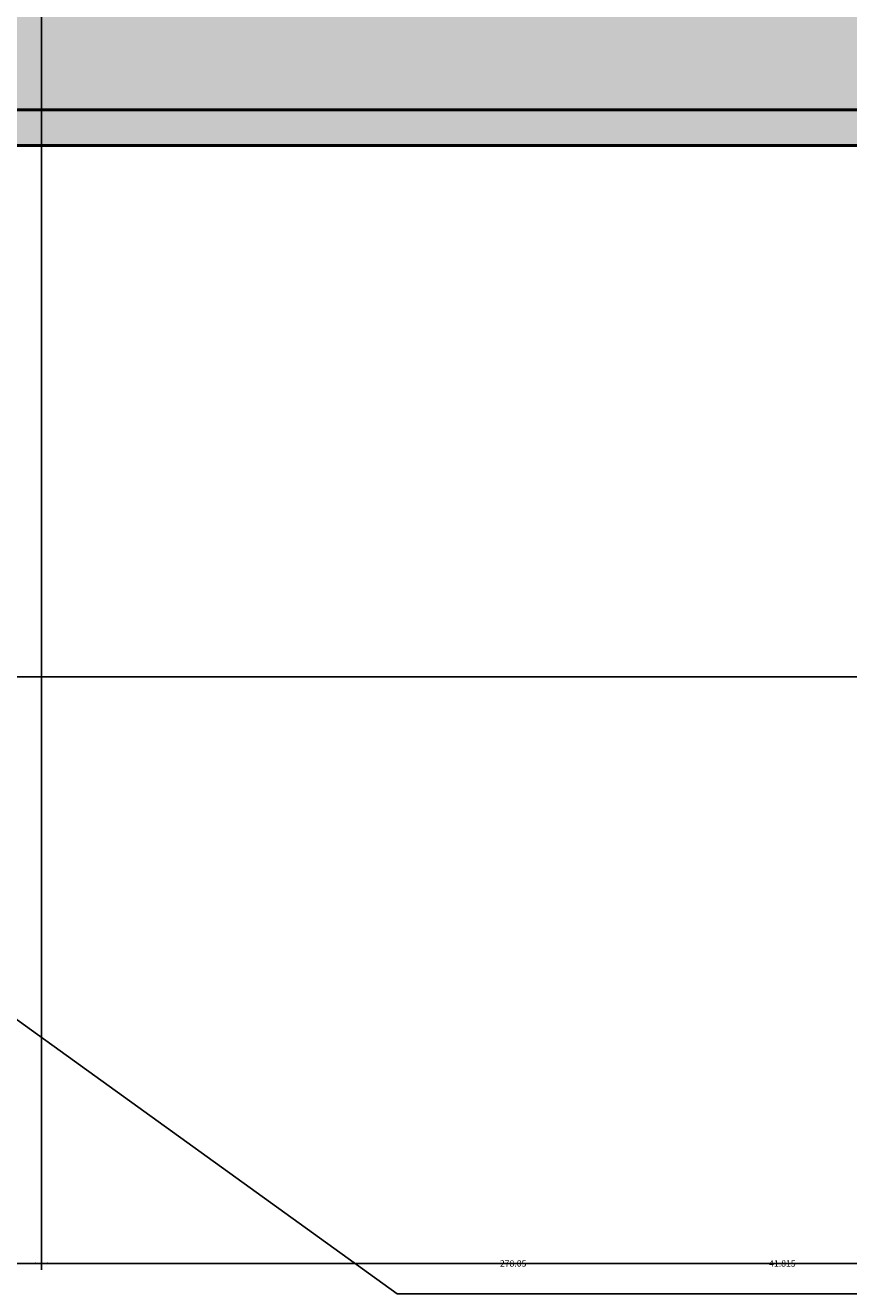
# Model space of a CAD drawing. Units: inches. Extents: x -12 to 334, y -10 to 186.
# Tile 31 of 77: x 129 to 152, y 14 to 49. Entities that reach past the tile are written whole.
import ezdxf
from ezdxf import colors
from ezdxf.entities.mleader import LeaderData, LeaderLine
from ezdxf.math import Vec2, Vec3

# ---------------------------------------------------------------- set-up
doc = ezdxf.new("R2010")
doc.units = ezdxf.units.IN
doc.header["$MEASUREMENT"] = 0
for name, color, linetype, lineweight in [('M-ANNO-TEXT', 3, 'Continuous', 25), ('M-DIMS', 2, 'Continuous', 18), ('M-EQPM', 7, 'Continuous', 50), ('M-EQPM-PATT', 8, 'Continuous', 18)]:
    doc.layers.add(name, color=color, linetype=linetype, lineweight=lineweight)
doc.styles.get("Standard").update_dxf_attribs({"font": 'arial.ttf'})
doc.dimstyles.get("Standard").update_dxf_attribs({"dimtxt": 0.18, "dimasz": 0.18, "dimexe": 0.18, "dimexo": 0.0625, "dimgap": 0.09, "dimtad": 0, "dimtih": 1, "dimtoh": 1, "dimdec": 4, "dimzin": 0, "dimdsep": 46, "dimtxsty": 'Standard', "dimcen": 0.09, "dimadec": 0, "dimazin": 0, "dimtfac": 1, "dimtdec": 4, "dimtofl": 0, "dimtmove": 0, "dimatfit": 3, "dimfxl": 1, "dimtolj": 1, "dimtzin": 0, "dimarcsym": 0})

# ---------------------------------------------------------------- blocks, each defined once
blk = doc.blocks.new('*D1')
at = {"layer": 'Defpoints', "color": 0, "transparency": 16777216}
for p in [(281.426, 91.899), (3.376, 80.692), (281.426, 14.304)]:
    blk.add_point(p, dxfattribs=at)
at = {"layer": 'M-DIMS', "color": 0, "lineweight": -2, "transparency": 16777216}
for p, q in [((281.426, 91.836), (281.426, 14.124)), ((3.376, 80.629), (3.376, 14.124)), ((3.556, 14.304), (141.935, 14.304)), ((281.246, 14.304), (142.867, 14.304))]:
    blk.add_line(p, q, dxfattribs=at)
at = {"layer": 'M-DIMS', "color": 0, "transparency": 16777216}
for points in [[(3.556, 14.334), (3.556, 14.274), (3.376, 14.304)], [(281.246, 14.334), (281.246, 14.274), (281.426, 14.304)]]:
    blk.add_solid(points, dxfattribs=at)
at = {"layer": 'M-DIMS', "color": 0, "transparency": 16777216, "insert": (142.401, 14.304), "char_height": 0.18, "attachment_point": 5}
blk.add_mtext('\\A1;278.05', dxfattribs=at)
blk = doc.blocks.new('*D29')
at = {"layer": 'Defpoints', "color": 0, "transparency": 16777216}
for p in [(-11.174, 45.854), (221.576, 45.854), (216.576, 30.854)]:
    blk.add_point(p, dxfattribs=at)
at = {"layer": 'M-DIMS', "color": 0, "lineweight": -2, "transparency": 16777216}
for p, q in [((221.514, 45.854), (-11.354, 45.854)), ((-11.174, 45.674), (-11.174, 38.536)), ((-11.174, 31.034), (-11.174, 38.172)), ((216.514, 30.854), (-11.354, 30.854))]:
    blk.add_line(p, q, dxfattribs=at)
at = {"layer": 'M-DIMS', "color": 0, "transparency": 16777216}
for points in [[(-11.204, 45.674), (-11.144, 45.674), (-11.174, 45.854)], [(-11.204, 31.034), (-11.144, 31.034), (-11.174, 30.854)]]:
    blk.add_solid(points, dxfattribs=at)
at = {"layer": 'M-DIMS', "color": 0, "transparency": 16777216, "insert": (-11.174, 38.354), "char_height": 0.18, "attachment_point": 5}
blk.add_mtext('\\A1;15', dxfattribs=at)
blk = doc.blocks.new('*D30')
at = {"layer": 'Defpoints', "color": 0, "transparency": 16777216}
for p in [(75.924, 63.612), (129.093, 61.105), (129.093, 14.304)]:
    blk.add_point(p, dxfattribs=at)
at = {"layer": 'M-DIMS', "color": 0, "lineweight": -2, "transparency": 16777216}
for p, q in [((75.924, 63.549), (75.924, 14.124)), ((129.093, 61.042), (129.093, 14.124)), ((76.104, 14.304), (102.115, 14.304)), ((128.913, 14.304), (102.902, 14.304))]:
    blk.add_line(p, q, dxfattribs=at)
at = {"layer": 'M-DIMS', "color": 0, "transparency": 16777216}
for points in [[(76.104, 14.334), (76.104, 14.274), (75.924, 14.304)], [(128.913, 14.334), (128.913, 14.274), (129.093, 14.304)]]:
    blk.add_solid(points, dxfattribs=at)
at = {"layer": 'M-DIMS', "color": 0, "transparency": 16777216, "insert": (102.509, 14.304), "char_height": 0.18, "attachment_point": 5}
blk.add_mtext('\\A1;53.17', dxfattribs=at)
blk = doc.blocks.new('*D31')
at = {"layer": 'Defpoints', "color": 0, "transparency": 16777216}
for p in [(129.093, 61.105), (170.908, 61.105), (170.908, 14.304)]:
    blk.add_point(p, dxfattribs=at)
at = {"layer": 'M-DIMS', "color": 0, "lineweight": -2, "transparency": 16777216}
for p, q in [((129.093, 61.042), (129.093, 14.124)), ((170.908, 61.042), (170.908, 14.124)), ((129.273, 14.304), (149.532, 14.304)), ((170.728, 14.304), (150.468, 14.304))]:
    blk.add_line(p, q, dxfattribs=at)
at = {"layer": 'M-DIMS', "color": 0, "transparency": 16777216}
for points in [[(129.273, 14.334), (129.273, 14.274), (129.093, 14.304)], [(170.728, 14.334), (170.728, 14.274), (170.908, 14.304)]]:
    blk.add_solid(points, dxfattribs=at)
at = {"layer": 'M-DIMS', "color": 0, "transparency": 16777216, "insert": (150, 14.304), "char_height": 0.18, "attachment_point": 5}
blk.add_mtext('\\A1;41.815', dxfattribs=at)
blk = doc.blocks.new('*D39')
at = {"layer": 'Defpoints', "color": 0, "transparency": 16777216}
for p in [(279.726, 80.692), (-11.174, 45.854), (269.381, 45.854)]:
    blk.add_point(p, dxfattribs=at)
at = {"layer": 'M-DIMS', "color": 0, "lineweight": -2, "transparency": 16777216}
for p, q in [((279.664, 80.692), (-11.354, 80.692)), ((-11.174, 80.512), (-11.174, 63.455)), ((-11.174, 46.034), (-11.174, 63.091)), ((269.318, 45.854), (-11.354, 45.854))]:
    blk.add_line(p, q, dxfattribs=at)
at = {"layer": 'M-DIMS', "color": 0, "transparency": 16777216}
for points in [[(-11.204, 80.512), (-11.144, 80.512), (-11.174, 80.692)], [(-11.204, 46.034), (-11.144, 46.034), (-11.174, 45.854)]]:
    blk.add_solid(points, dxfattribs=at)
at = {"layer": 'M-DIMS', "color": 0, "transparency": 16777216, "insert": (-11.174, 63.273), "char_height": 0.18, "attachment_point": 5}
blk.add_mtext('\\A1;34.84', dxfattribs=at)

msp = doc.modelspace()

# ---------------------------------------------------------------- hatches: boundary and pattern name
at = {"layer": 'M-EQPM-PATT'}
h = msp.add_hatch(color=256, dxfattribs=at)
h.set_gradient(color1=(99, 100, 102), color2=(99, 100, 102), tint=1)
h.paths.add_polyline_path([(4.3766, 80.754, -0.4132606), (23.5807, 99.8958), (37.1002, 99.8958), (37.1002, 127.7078), (32.1002, 127.7078), (32.1002, 125.2078), (36.1002, 125.2078), (36.1002, 100.8958), (23.5807, 100.8958, 1), (23.5807, 60.4872), (36.1002, 60.4872), (36.1002, 36.1752), (32.1002, 36.1752), (32.1002, 33.6752), (37.1002, 33.6752), (37.1002, 61.4872), (23.5807, 61.4872, -0.384914), (4.4744, 78.754), (72.9244, 78.754), (72.9244, 69.6117), (75.9244, 69.6117), (75.9244, 89.8963), (72.9244, 89.8963), (72.9244, 80.754)])
h.paths.add_polyline_path([(54.1002, 125.2078), (58.1002, 125.2078), (58.1002, 127.7078), (53.1002, 127.7078), (53.1002, 99.8958), (64.5, 99.8958), (64.5, 109.0583), (63.5, 109.0583), (63.5, 100.8958), (54.1002, 100.8958)], flags=17)
h.paths.add_polyline_path([(53.1002, 33.6752), (58.1002, 33.6752), (58.1002, 36.1752), (54.1002, 36.1752), (54.1002, 60.4872), (64.2068, 60.4872), (64.2068, 49.4497), (87.8879, 49.4497), (87.8879, 55.3205), (104.8919, 55.3205), (104.8919, 30.8541), (99.8919, 30.8541), (99.8919, 28.8541), (105.8919, 28.8541), (105.8919, 56.3205), (87.8879, 56.3205), (87.8879, 63.6117), (86.8879, 63.6117), (86.8879, 50.4497), (65.0061, 50.4497), (65.0061, 63.6117), (64.5, 63.6117), (64.5, 61.4872), (53.1002, 61.4872)])
h.paths.add_polyline_path([(121.8919, 28.8541), (121.8919, 30.8541), (116.8919, 30.8541), (116.8919, 45.8541), (209.6965, 45.8541), (209.9204, 46.8541), (115.8919, 46.8541), (115.8919, 28.8541)])
h.paths.add_polyline_path([(221.5761, 32.8541), (216.5761, 32.8541), (216.5761, 30.8541), (222.5761, 30.8541), (222.5761, 46.8541), (209.9204, 46.8541), (209.6965, 45.8541), (221.5761, 45.8541)])
h.paths.add_polyline_path([(233.5761, 45.8541), (249.8485, 45.8541), (249.3759, 46.8541), (232.5761, 46.8541), (232.5761, 30.8541), (238.5761, 30.8541), (238.5761, 32.8541), (233.5761, 32.8541)])
h = msp.add_hatch(color=256, dxfattribs=at)
h.set_gradient(color1=(94, 103, 175), color2=(94, 103, 175), tint=1)
h.paths.add_polyline_path([(129.093, 89.8963), (86.8879, 89.8963), (86.8879, 69.6117), (129.093, 69.6117)], flags=17)
h.paths.add_polyline_path([(170.9079, 89.8963), (130.8573, 89.8963), (130.8573, 69.6117), (170.9079, 69.6117)], flags=17)
h.paths.add_polyline_path([(216.4278, 89.8963), (172.6722, 89.8963), (172.6722, 69.6117), (216.4278, 69.6117)], flags=17)
h.paths.add_polyline_path([(245.9354, 82.6969), (247.9354, 82.6969), (247.9354, 46.8541), (268.3808, 46.8541, 0.0998398), (279.7263, 80.6915), (251.9801, 80.6915, 0.4142136), (231.7758, 100.8958), (84.7229, 100.8958), (84.7229, 109.0583), (83.7229, 109.0583), (83.7229, 95.8963), (129.093, 95.8963), (129.093, 98.1081), (130.8573, 98.1081), (130.8573, 95.8963), (170.9079, 95.8963), (170.9079, 98.1081), (172.6722, 98.1081), (172.6722, 95.8963), (216.4278, 95.8963), (216.4278, 98.1081), (218.1922, 98.1081), (218.1922, 95.8963), (226.6083, 95.8963, -1), (226.6083, 63.6117), (218.1922, 63.6117), (218.1922, 61.1045), (216.4278, 61.1045), (216.4278, 63.6117), (172.6722, 63.6117), (172.6722, 61.1045), (170.9079, 61.1045), (170.9079, 63.6117), (130.8573, 63.6117), (130.8573, 61.1045), (129.093, 61.1045), (129.093, 63.6117), (87.8879, 63.6117), (87.8879, 56.3205), (105.8919, 56.3205), (105.8919, 28.8541), (115.8919, 28.8541), (115.8919, 46.8541), (222.5761, 46.8541), (222.5761, 30.8541), (232.5761, 30.8541), (232.5761, 46.8541), (245.9354, 46.8541)])
h.paths.add_polyline_path([(86.8879, 89.8963), (75.9244, 89.8963), (75.9244, 69.6117), (86.8879, 69.6117)])
h.paths.add_polyline_path([(83.7229, 109.0583), (75.9244, 109.0583), (75.9244, 95.8963), (83.7229, 95.8963)])
h.paths.add_polyline_path([(226.6083, 89.8963), (218.1922, 89.8963), (218.1922, 69.6117), (226.6083, 69.6117, 1)], flags=17)
h = msp.add_hatch(color=256, dxfattribs=at)
h.set_gradient(color1=(0, 0, 255), color2=(0, 0, 255), tint=1)
h.paths.add_polyline_path([(84.7229, 100.8958), (84.7229, 109.0583), (83.7229, 109.0583), (83.7229, 95.8963), (129.093, 95.8963), (129.093, 98.1081), (130.8573, 98.1081), (130.8573, 95.8963), (170.9079, 95.8963), (170.9079, 98.1081), (172.6722, 98.1081), (172.6722, 95.8963), (216.4278, 95.8963), (216.4278, 98.1081), (218.1922, 98.1081), (218.1922, 95.8963), (226.6083, 95.8963, -1), (226.6083, 63.6117), (218.1922, 63.6117), (218.1922, 61.1045), (216.4278, 61.1045), (216.4278, 63.6117), (172.6722, 63.6117), (172.6722, 61.1045), (170.9079, 61.1045), (170.9079, 63.6117), (130.8573, 63.6117), (130.8573, 61.1045), (129.093, 61.1045), (129.093, 63.6117), (87.8879, 63.6117), (87.8879, 56.3205), (105.8919, 56.3205), (105.8919, 28.8541), (115.8919, 28.8541), (115.8919, 46.8541), (222.5761, 46.8541), (222.5761, 30.8541), (232.5761, 30.8541), (232.5761, 46.8541), (245.9354, 46.8541), (245.9354, 82.6969), (247.9354, 82.6969), (247.9354, 46.8541), (268.3808, 46.8541, 0.0998398), (279.7263, 80.6915), (251.9801, 80.6915, 0.4142136), (231.7758, 100.8958)])

# ---------------------------------------------------------------- linework, layer by layer
at = {"layer": 'M-EQPM'}
for p, q in [((222.5761, 46.8541), (115.8919, 46.8541)), ((221.5761, 45.8541), (116.8919, 45.8541))]:
    msp.add_line(p, q, dxfattribs=at)

# ---------------------------------------------------------------- dimensions: what is measured, and where the dimension line sits
at = {"layer": 'M-DIMS'}
for base, p1, p2, override, picture, middle in [((281.4256, 14.3041), (3.3765, 80.6915), (281.4256, 91.8988), {"dimdec": 2, "dimlfac": 1, "dimrnd": 0, "dimzin": 0, "dimdsep": 46, "dimlunit": 2}, '*D1', (142.401, 14.3041)), ((129.093, 14.3041), (75.9244, 63.6117), (129.093, 61.1045), {"dimdec": 2, "dimlfac": 1, "dimrnd": 0, "dimzin": 0, "dimdsep": 46, "dimlunit": 2}, '*D30', (102.5087, 14.3041)), ((170.9079, 14.3041), (129.093, 61.1045), (170.9079, 61.1045), {"dimdec": 3, "dimlfac": 1, "dimrnd": 0, "dimzin": 0, "dimdsep": 46, "dimlunit": 2}, '*D31', (150.0004, 14.3041))]:
    dim = msp.add_linear_dim(base=base, p1=p1, p2=p2, dimstyle='Standard', override=override, dxfattribs=at)
    dim.commit()
    dim.dimension.update_dxf_attribs({"geometry": picture, "text_midpoint": middle})
for p1, p2, override, picture, middle in [((279.7263, 80.6915), (269.3808, 45.8541), {"dimdec": 2, "dimlfac": 1, "dimrnd": 0, "dimzin": 0, "dimdsep": 46, "dimlunit": 2}, '*D39', (-11.1735, 63.2728)), ((216.5761, 30.8541), (221.5761, 45.8541), {"dimdec": 0, "dimlfac": 1, "dimrnd": 0, "dimzin": 0, "dimdsep": 46, "dimlunit": 2}, '*D29', (-11.1735, 38.3541))]:
    dim = msp.add_linear_dim(base=(-11.1736, 45.8541), p1=p1, p2=p2, angle=90, dimstyle='Standard', override=override, dxfattribs=at)
    dim.commit()
    dim.dimension.update_dxf_attribs({"geometry": picture, "text_midpoint": middle})

# ---------------------------------------------------------------- leaders
at = {"layer": 'M-ANNO-TEXT'}
ml = msp.add_multileader_mtext('Standard', dxfattribs=at)
ml.set_content('^ICondensate outlet', color=256)
ml.set_leader_properties()
ml.build(insert=Vec2(0, 0))
ml.multileader.update_dxf_attribs({"dogleg_length": 0.36, "arrow_head_size": 0.7})
ctx = ml.context
ctx.base_point, ctx.arrow_head_size, ctx.landing_gap_size, ctx.plane_origin = Vec3(83.8784, 10.3512), 0.7, 0.09, Vec3(49.4251, 25.7584)
notes = []
notes.append((ctx, [(0, (1, 1, 0), (70.8242, 10.3512), (1, 0), 13.0542, [(0, [(42.9275, 33.6752)], 0, [])])]))
ctx.mtext.insert, ctx.mtext.flow_direction = Vec3(83.9684, 12.3853), 5
ml = msp.add_multileader_mtext('Standard', dxfattribs=at)
ml.set_content('liquid feed from\\Pcolumn', color=256)
ml.set_leader_properties()
ml.build(insert=Vec2(0, 0))
ml.multileader.update_dxf_attribs({"dogleg_length": 0.36, "arrow_head_size": 0.7})
ctx = ml.context
ctx.base_point, ctx.arrow_head_size, ctx.landing_gap_size, ctx.plane_origin = Vec3(152.1867, 13.4469), 0.7, 0.09, Vec3(117.7335, 28.8541)
notes.append((ctx, [(0, (1, 1, 0), (139.1325, 13.4469), (1, 0), 13.0542, [(0, [(117.7335, 28.8541)], 0, [])])]))
ctx.mtext.insert, ctx.mtext.flow_direction = Vec3(152.2767, 15.4796), 5
for ctx, leaders in notes:
    for number, flags, end, landing, length, lines in leaders:
        leader = LeaderData()
        leader.index, (leader.has_last_leader_line, leader.has_dogleg_vector, leader.attachment_direction) = number, flags
        leader.last_leader_point, leader.dogleg_vector, leader.dogleg_length = Vec3(end), Vec3(landing), length
        for number, points, colour, breaks in lines:
            line = LeaderLine()
            line.index, line.vertices, line.color, line.breaks = number, Vec3.list(points), colors.encode_raw_color(colour), breaks
            leader.lines.append(line)
        ctx.leaders.append(leader)

doc.saveas('drawing.dxf')
